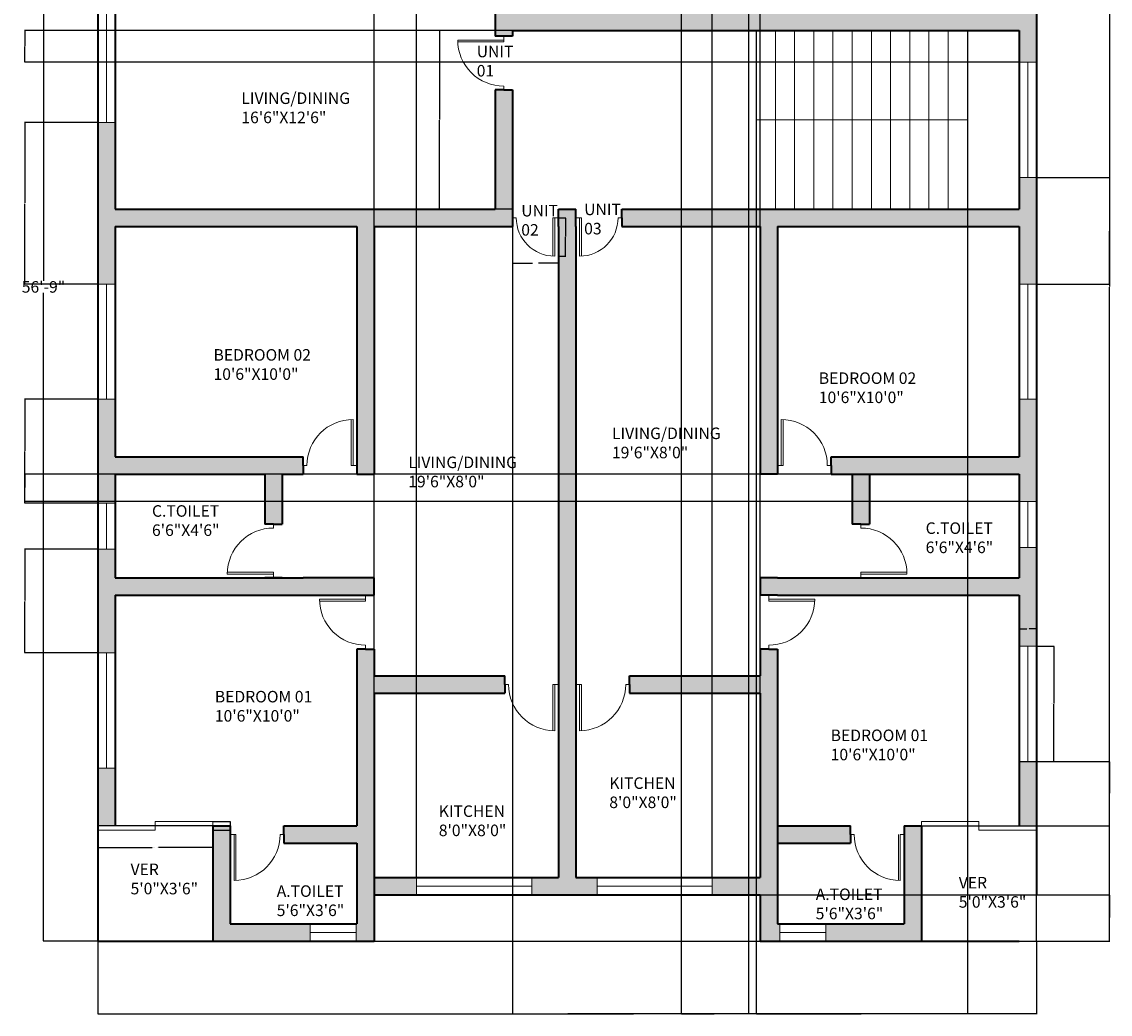
# Model space of a CAD drawing. Units: inches. Extents: x -17 to 550, y -704 to 87.
# Tile 1 of 2: x -17 to 550, y -704 to -187. Entities that reach past the tile are written whole.
import ezdxf

# ---------------------------------------------------------------- set-up
doc = ezdxf.new("R2010")
doc.units = ezdxf.units.IN
doc.header["$MEASUREMENT"] = 0
for name, color, linetype, lineweight in [('A-ANNO-DIMS', 2, 'Continuous', 18), ('A-AREA-IDEN', 7, 'Continuous', 18), ('A-DOOR', 3, 'Continuous', 18), ('A-FLOR-OTLN', 7, 'Continuous', 25), ('A-FLOR-STRS', 7, 'Continuous', 18), ('A-GLAZ', 4, 'Continuous', 18), ('A-WALL', 7, 'Continuous', 35), ('A-WALL-PATT', 252, 'Continuous', 13)]:
    doc.layers.add(name, color=color, linetype=linetype, lineweight=lineweight)
doc.styles.get("Standard").update_dxf_attribs({"font": 'arial.ttf'})
doc.dimstyles.get("Standard").update_dxf_attribs({"dimtxt": 0.18, "dimasz": 0.18, "dimexe": 0.18, "dimexo": 0.0625, "dimgap": 0.09, "dimtad": 0, "dimtih": 1, "dimtoh": 1, "dimdec": 0, "dimzin": 0, "dimdsep": 46, "dimlunit": 3, "dimtxsty": 'Standard', "dimcen": 0.09, "dimadec": 0, "dimazin": 0, "dimtfac": 1, "dimtdec": 0, "dimtofl": 0, "dimtmove": 0, "dimatfit": 3, "dimfxl": 1, "dimtolj": 1, "dimtzin": 0, "dimarcsym": 0})

# ---------------------------------------------------------------- blocks, each defined once
blk = doc.blocks.new('*D2')
at = {"layer": 'A-ANNO-DIMS', "color": 0, "lineweight": -2, "transparency": 16777216}
for p, q in [((22.68, 15.33), (-5.69, 15.33)), ((-5.51, 15.15), (-5.51, -322.02)), ((-5.51, -665.49), (-5.51, -328.33)), ((22.68, -665.67), (-5.69, -665.67))]:
    blk.add_line(p, q, dxfattribs=at)
at = {"layer": 'A-ANNO-DIMS', "color": 0, "transparency": 16777216}
for points in [[(-5.54, 15.15), (-5.48, 15.15), (-5.51, 15.33)], [(-5.54, -665.49), (-5.48, -665.49), (-5.51, -665.67)]]:
    blk.add_solid(points, dxfattribs=at)
at = {"layer": 'Defpoints', "color": 0, "transparency": 16777216}
for p in [(22.74, 15.33), (-5.51, -665.67), (22.74, -665.67)]:
    blk.add_point(p, dxfattribs=at)
at = {"layer": 'A-ANNO-DIMS', "color": 0, "transparency": 16777216, "insert": (-5.51, -325.17), "char_height": 6, "attachment_point": 5}
blk.add_mtext('\\A1;56\'-9"', dxfattribs=at)
blk = doc.blocks.new('WIN-60IN')
for p, q in [((0, 9), (60, 9)), ((0, 0), (0, 9)), ((60, 9), (60, 0)), ((0, 4.5), (60, 4.5)), ((60, 0), (0, 0))]:
    blk.add_line(p, q)
blk = doc.blocks.new('WIN-24IN')
for p, q in [((0, 24), (0, 0)), ((9, 24), (0, 24)), ((4.5, 24), (4.5, 0)), ((9, 0), (9, 24)), ((0, 0), (9, 0))]:
    blk.add_line(p, q)
blk = doc.blocks.new('DOOR-SWING-24IN')
for p, q in [((25, 0), (25, 24)), ((26, 0), (26, 24)), ((2, 0), (0, 0)), ((25, 0), (26, 0)), ((28, 0), (26, 0))]:
    blk.add_line(p, q)
blk.add_arc((26, 0), 24, 90, 180)
blk = doc.blocks.new('DOOR-SWING-20IN')
for p, q in [((0, 20), (2, 20)), ((21, 20), (21, 0)), ((21, 20), (22, 20)), ((22, 20), (22, 0)), ((24, 20), (22, 20))]:
    blk.add_line(p, q)
blk.add_arc((22, 20), 20, 180, 270)
blk = doc.blocks.new('DOOR-SLIDING-60IN')
for p, q in [((0, 0), (0, 2.25)), ((0, 2.25), (60, 2.25)), ((30, 4.5), (60, 4.5)), ((30, 2.25), (30, 4.5)), ((30, 2.25), (30, 0)), ((60, 4.5), (60, 2.25)), ((30, 0), (0, 0))]:
    blk.add_line(p, q)
blk = doc.blocks.new('*D10')
at = {"layer": 'A-ANNO-DIMS', "color": 0, "lineweight": -2, "transparency": 16777216}
for p, q in [((511.81, -512.17), (520.92, -512.17)), ((520.74, -512.35), (520.74, -541.99)), ((520.74, -571.99), (520.74, -542.36)), ((511.81, -572.17), (520.92, -572.17))]:
    blk.add_line(p, q, dxfattribs=at)
at = {"layer": 'A-ANNO-DIMS', "color": 0, "transparency": 16777216}
for points in [[(520.71, -512.35), (520.77, -512.35), (520.74, -512.17)], [(520.71, -571.99), (520.77, -571.99), (520.74, -572.17)]]:
    blk.add_solid(points, dxfattribs=at)
at = {"layer": 'Defpoints', "color": 0, "transparency": 16777216}
for p in [(511.74, -512.17), (520.74, -512.17), (511.74, -572.17)]:
    blk.add_point(p, dxfattribs=at)
at = {"layer": 'A-ANNO-DIMS', "color": 0, "transparency": 16777216, "insert": (520.74, -542.17), "char_height": 0.18, "attachment_point": 5}
blk.add_mtext('\\A1;WINDOW 5\'-0" TYP.', dxfattribs=at)
blk = doc.blocks.new('*D11')
at = {"layer": 'A-ANNO-DIMS', "color": 0, "lineweight": -2, "transparency": 16777216}
for p, q in [((502.74, -512.11), (502.74, -502.99)), ((502.92, -503.17), (506.6, -503.17)), ((511.56, -503.17), (507.88, -503.17)), ((511.74, -512.11), (511.74, -502.99))]:
    blk.add_line(p, q, dxfattribs=at)
at = {"layer": 'A-ANNO-DIMS', "color": 0, "transparency": 16777216}
for points in [[(502.92, -503.14), (502.92, -503.2), (502.74, -503.17)], [(511.56, -503.14), (511.56, -503.2), (511.74, -503.17)]]:
    blk.add_solid(points, dxfattribs=at)
at = {"layer": 'Defpoints', "color": 0, "transparency": 16777216}
for p in [(502.74, -503.17), (502.74, -512.17), (511.74, -512.17)]:
    blk.add_point(p, dxfattribs=at)
at = {"layer": 'A-ANNO-DIMS', "color": 0, "transparency": 16777216, "insert": (507.24, -503.17), "char_height": 0.18, "attachment_point": 5}
blk.add_mtext('\\A1;0\'-9" TYP.', dxfattribs=at)
blk = doc.blocks.new('*D14')
at = {"layer": 'A-ANNO-DIMS', "color": 0, "lineweight": -2, "transparency": 16777216}
for p, q in [((238.74, -309.24), (238.74, -312.95)), ((262.74, -309.24), (262.74, -312.95)), ((238.92, -312.77), (249.24, -312.77)), ((262.56, -312.77), (252.25, -312.77))]:
    blk.add_line(p, q, dxfattribs=at)
at = {"layer": 'A-ANNO-DIMS', "color": 0, "transparency": 16777216}
for points in [[(238.92, -312.74), (238.92, -312.8), (238.74, -312.77)], [(262.56, -312.74), (262.56, -312.8), (262.74, -312.77)]]:
    blk.add_solid(points, dxfattribs=at)
at = {"layer": 'Defpoints', "color": 0, "transparency": 16777216}
for p in [(238.74, -309.17), (262.74, -309.17), (262.74, -312.77)]:
    blk.add_point(p, dxfattribs=at)
at = {"layer": 'A-ANNO-DIMS', "color": 0, "transparency": 16777216, "insert": (250.74, -312.77), "char_height": 0.18, "attachment_point": 5}
blk.add_mtext('\\A1;ENTRY DOOR 2\'-0" TYP.', dxfattribs=at)
blk = doc.blocks.new('*D15')
at = {"layer": 'A-ANNO-DIMS', "color": 0, "lineweight": -2, "transparency": 16777216}
for p, q in [((262.81, -289.17), (266.52, -289.17)), ((266.34, -289.35), (266.34, -298.99)), ((266.34, -308.99), (266.34, -299.36)), ((262.81, -309.17), (266.52, -309.17))]:
    blk.add_line(p, q, dxfattribs=at)
at = {"layer": 'A-ANNO-DIMS', "color": 0, "transparency": 16777216}
for points in [[(266.31, -289.35), (266.37, -289.35), (266.34, -289.17)], [(266.31, -308.99), (266.37, -308.99), (266.34, -309.17)]]:
    blk.add_solid(points, dxfattribs=at)
at = {"layer": 'Defpoints', "color": 0, "transparency": 16777216}
for p in [(262.74, -289.17), (266.34, -289.17), (262.74, -309.17)]:
    blk.add_point(p, dxfattribs=at)
at = {"layer": 'A-ANNO-DIMS', "color": 0, "transparency": 16777216, "insert": (266.34, -299.17), "char_height": 0.18, "attachment_point": 5}
blk.add_mtext('\\A1;1\'-8" TYP.', dxfattribs=at)
blk = doc.blocks.new('*D16')
at = {"layer": 'A-ANNO-DIMS', "color": 0, "lineweight": -2, "transparency": 16777216}
for p, q in [((22.74, -607.99), (22.74, -617.1)), ((82.74, -607.99), (82.74, -617.1)), ((22.92, -616.92), (51.15, -616.92)), ((82.56, -616.92), (54.33, -616.92))]:
    blk.add_line(p, q, dxfattribs=at)
at = {"layer": 'A-ANNO-DIMS', "color": 0, "transparency": 16777216}
for points in [[(22.92, -616.89), (22.92, -616.95), (22.74, -616.92)], [(82.56, -616.89), (82.56, -616.95), (82.74, -616.92)]]:
    blk.add_solid(points, dxfattribs=at)
at = {"layer": 'Defpoints', "color": 0, "transparency": 16777216}
for p in [(22.74, -607.92), (82.74, -607.92), (82.74, -616.92)]:
    blk.add_point(p, dxfattribs=at)
at = {"layer": 'A-ANNO-DIMS', "color": 0, "transparency": 16777216, "insert": (52.74, -616.92), "char_height": 0.18, "attachment_point": 5}
blk.add_mtext('\\A1;SLIDING DOOR 5\'-0" TYP.', dxfattribs=at)
blk = doc.blocks.new('*D17')
at = {"layer": 'A-ANNO-DIMS', "color": 0, "lineweight": -2, "transparency": 16777216}
for p, q in [((82.81, -603.42), (91.92, -603.42)), ((91.74, -603.6), (91.74, -605.49)), ((91.74, -607.74), (91.74, -605.86)), ((82.81, -607.92), (91.92, -607.92))]:
    blk.add_line(p, q, dxfattribs=at)
at = {"layer": 'A-ANNO-DIMS', "color": 0, "transparency": 16777216}
for points in [[(91.71, -603.6), (91.77, -603.6), (91.74, -603.42)], [(91.71, -607.74), (91.77, -607.74), (91.74, -607.92)]]:
    blk.add_solid(points, dxfattribs=at)
at = {"layer": 'Defpoints', "color": 0, "transparency": 16777216}
for p in [(82.74, -603.42), (91.74, -603.42), (82.74, -607.92)]:
    blk.add_point(p, dxfattribs=at)
at = {"layer": 'A-ANNO-DIMS', "color": 0, "transparency": 16777216, "insert": (91.74, -605.67), "char_height": 0.18, "attachment_point": 5}
blk.add_mtext('\\A1;0\'-4 1/2" TYP.', dxfattribs=at)
blk = doc.blocks.new('*D18')
at = {"layer": 'A-ANNO-DIMS', "color": 0, "lineweight": -2, "transparency": 16777216}
for p, q in [((22.74, -665.74), (22.74, -703.75)), ((511.74, -665.74), (511.74, -703.75)), ((22.92, -703.57), (266.84, -703.57)), ((511.56, -703.57), (267.65, -703.57))]:
    blk.add_line(p, q, dxfattribs=at)
at = {"layer": 'A-ANNO-DIMS', "color": 0, "transparency": 16777216}
for points in [[(22.92, -703.54), (22.92, -703.6), (22.74, -703.57)], [(511.56, -703.54), (511.56, -703.6), (511.74, -703.57)]]:
    blk.add_solid(points, dxfattribs=at)
at = {"layer": 'Defpoints', "color": 0, "transparency": 16777216}
for p in [(22.74, -665.67), (511.74, -665.67), (511.74, -703.57)]:
    blk.add_point(p, dxfattribs=at)
at = {"layer": 'A-ANNO-DIMS', "color": 0, "transparency": 16777216, "insert": (267.24, -703.57), "char_height": 0.18, "attachment_point": 5}
blk.add_mtext('\\A1;40\'-9"', dxfattribs=at)
blk = doc.blocks.new('*D19')
at = {"layer": 'A-ANNO-DIMS', "color": 0, "lineweight": -2, "transparency": 16777216}
for p, q in [((238.68, -191.67), (200.66, -191.67)), ((200.84, -191.85), (200.84, -237.99)), ((200.84, -284.49), (200.84, -238.36)), ((238.68, -284.67), (200.66, -284.67))]:
    blk.add_line(p, q, dxfattribs=at)
at = {"layer": 'A-ANNO-DIMS', "color": 0, "transparency": 16777216}
for points in [[(200.81, -191.85), (200.87, -191.85), (200.84, -191.67)], [(200.81, -284.49), (200.87, -284.49), (200.84, -284.67)]]:
    blk.add_solid(points, dxfattribs=at)
at = {"layer": 'Defpoints', "color": 0, "transparency": 16777216}
for p in [(200.84, -191.67), (238.74, -191.67), (238.74, -284.67)]:
    blk.add_point(p, dxfattribs=at)
at = {"layer": 'A-ANNO-DIMS', "color": 0, "transparency": 16777216, "insert": (200.84, -238.17), "char_height": 0.18, "attachment_point": 5}
blk.add_mtext('\\A1;7\'-9"', dxfattribs=at)
blk = doc.blocks.new('*D20')
at = {"layer": 'A-ANNO-DIMS', "color": 0, "lineweight": -2, "transparency": 16777216}
for p, q in [((365.68, -191.74), (365.68, -703.75)), ((475.68, -191.74), (475.68, -703.75)), ((365.86, -703.57), (420.35, -703.57)), ((475.5, -703.57), (421.01, -703.57))]:
    blk.add_line(p, q, dxfattribs=at)
at = {"layer": 'A-ANNO-DIMS', "color": 0, "transparency": 16777216}
for points in [[(365.86, -703.54), (365.86, -703.6), (365.68, -703.57)], [(475.5, -703.54), (475.5, -703.6), (475.68, -703.57)]]:
    blk.add_solid(points, dxfattribs=at)
at = {"layer": 'Defpoints', "color": 0, "transparency": 16777216}
for p in [(365.68, -191.67), (475.68, -191.67), (475.68, -703.57)]:
    blk.add_point(p, dxfattribs=at)
at = {"layer": 'A-ANNO-DIMS', "color": 0, "transparency": 16777216, "insert": (420.68, -703.57), "char_height": 0.18, "attachment_point": 5}
blk.add_mtext('\\A1;9\'-2"', dxfattribs=at)
blk = doc.blocks.new('*D21')
at = {"layer": 'A-ANNO-DIMS', "color": 0, "lineweight": -2, "transparency": 16777216}
for p, q in [((238.74, -222.74), (238.74, -703.75)), ((365.68, -238.24), (365.68, -703.75)), ((238.92, -703.57), (301.82, -703.57)), ((365.5, -703.57), (302.6, -703.57))]:
    blk.add_line(p, q, dxfattribs=at)
at = {"layer": 'A-ANNO-DIMS', "color": 0, "transparency": 16777216}
for points in [[(238.92, -703.54), (238.92, -703.6), (238.74, -703.57)], [(365.5, -703.54), (365.5, -703.6), (365.68, -703.57)]]:
    blk.add_solid(points, dxfattribs=at)
at = {"layer": 'Defpoints', "color": 0, "transparency": 16777216}
for p in [(238.74, -222.67), (365.68, -238.17), (365.68, -703.57)]:
    blk.add_point(p, dxfattribs=at)
at = {"layer": 'A-ANNO-DIMS', "color": 0, "transparency": 16777216, "insert": (302.21, -703.57), "char_height": 0.18, "attachment_point": 5}
blk.add_mtext('\\A1;10\'-7"', dxfattribs=at)
blk = doc.blocks.new('*D22')
at = {"layer": 'A-ANNO-DIMS', "color": 0, "lineweight": -2, "transparency": 16777216}
for p, q in [((166.81, -641.67), (549.82, -641.67)), ((549.64, -641.85), (549.64, -653.49)), ((549.64, -665.49), (549.64, -653.86)), ((166.81, -665.67), (549.82, -665.67))]:
    blk.add_line(p, q, dxfattribs=at)
at = {"layer": 'A-ANNO-DIMS', "color": 0, "transparency": 16777216}
for points in [[(549.61, -641.85), (549.67, -641.85), (549.64, -641.67)], [(549.61, -665.49), (549.67, -665.49), (549.64, -665.67)]]:
    blk.add_solid(points, dxfattribs=at)
at = {"layer": 'Defpoints', "color": 0, "transparency": 16777216}
for p in [(166.74, -641.67), (549.64, -641.67), (166.74, -665.67)]:
    blk.add_point(p, dxfattribs=at)
at = {"layer": 'A-ANNO-DIMS', "color": 0, "transparency": 16777216, "insert": (549.64, -653.67), "char_height": 0.18, "attachment_point": 5}
blk.add_mtext('\\A1;2\'-0"', dxfattribs=at)
blk = doc.blocks.new('*D29')
at = {"layer": 'A-ANNO-DIMS', "color": 0, "lineweight": -2, "transparency": 16777216}
for p, q in [((22.68, -239.67), (-15.34, -239.67)), ((-15.16, -239.85), (-15.16, -281.49)), ((-15.16, -323.49), (-15.16, -281.86)), ((22.68, -323.67), (-15.34, -323.67))]:
    blk.add_line(p, q, dxfattribs=at)
at = {"layer": 'A-ANNO-DIMS', "color": 0, "transparency": 16777216}
for points in [[(-15.19, -239.85), (-15.13, -239.85), (-15.16, -239.67)], [(-15.19, -323.49), (-15.13, -323.49), (-15.16, -323.67)]]:
    blk.add_solid(points, dxfattribs=at)
at = {"layer": 'Defpoints', "color": 0, "transparency": 16777216}
for p in [(-15.16, -239.67), (22.74, -239.67), (22.74, -323.67)]:
    blk.add_point(p, dxfattribs=at)
at = {"layer": 'A-ANNO-DIMS', "color": 0, "transparency": 16777216, "insert": (-15.16, -281.67), "char_height": 0.18, "attachment_point": 5}
blk.add_mtext('\\A1;7\'-0"', dxfattribs=at)
blk = doc.blocks.new('*D30')
at = {"layer": 'A-ANNO-DIMS', "color": 0, "lineweight": -2, "transparency": 16777216}
for p, q in [((22.68, -383.67), (-15.34, -383.67)), ((-15.16, -383.85), (-15.16, -410.49)), ((-15.16, -437.49), (-15.16, -410.86)), ((22.68, -437.67), (-15.34, -437.67))]:
    blk.add_line(p, q, dxfattribs=at)
at = {"layer": 'A-ANNO-DIMS', "color": 0, "transparency": 16777216}
for points in [[(-15.19, -383.85), (-15.13, -383.85), (-15.16, -383.67)], [(-15.19, -437.49), (-15.13, -437.49), (-15.16, -437.67)]]:
    blk.add_solid(points, dxfattribs=at)
at = {"layer": 'Defpoints', "color": 0, "transparency": 16777216}
for p in [(-15.16, -383.67), (22.74, -383.67), (22.74, -437.67)]:
    blk.add_point(p, dxfattribs=at)
at = {"layer": 'A-ANNO-DIMS', "color": 0, "transparency": 16777216, "insert": (-15.16, -410.67), "char_height": 0.18, "attachment_point": 5}
blk.add_mtext('\\A1;4\'-6"', dxfattribs=at)
blk = doc.blocks.new('*D31')
at = {"layer": 'A-ANNO-DIMS', "color": 0, "lineweight": -2, "transparency": 16777216}
for p, q in [((22.68, -461.67), (-15.34, -461.67)), ((-15.16, -461.85), (-15.16, -488.49)), ((-15.16, -515.49), (-15.16, -488.86)), ((22.68, -515.67), (-15.34, -515.67))]:
    blk.add_line(p, q, dxfattribs=at)
at = {"layer": 'A-ANNO-DIMS', "color": 0, "transparency": 16777216}
for points in [[(-15.19, -461.85), (-15.13, -461.85), (-15.16, -461.67)], [(-15.19, -515.49), (-15.13, -515.49), (-15.16, -515.67)]]:
    blk.add_solid(points, dxfattribs=at)
at = {"layer": 'Defpoints', "color": 0, "transparency": 16777216}
for p in [(-15.16, -461.67), (22.74, -461.67), (22.74, -515.67)]:
    blk.add_point(p, dxfattribs=at)
at = {"layer": 'A-ANNO-DIMS', "color": 0, "transparency": 16777216, "insert": (-15.16, -488.67), "char_height": 0.18, "attachment_point": 5}
blk.add_mtext('\\A1;4\'-6"', dxfattribs=at)
blk = doc.blocks.new('*D32')
at = {"layer": 'A-ANNO-DIMS', "color": 0, "lineweight": -2, "transparency": 16777216}
for p, q in [((326.67, -134.74), (326.67, -703.75)), ((361.74, -134.74), (361.74, -703.75)), ((326.85, -703.57), (343.81, -703.57)), ((361.56, -703.57), (344.61, -703.57))]:
    blk.add_line(p, q, dxfattribs=at)
at = {"layer": 'A-ANNO-DIMS', "color": 0, "transparency": 16777216}
for points in [[(326.85, -703.54), (326.85, -703.6), (326.67, -703.57)], [(361.56, -703.54), (361.56, -703.6), (361.74, -703.57)]]:
    blk.add_solid(points, dxfattribs=at)
at = {"layer": 'Defpoints', "color": 0, "transparency": 16777216}
for p in [(326.67, -134.67), (361.74, -134.67), (361.74, -703.57)]:
    blk.add_point(p, dxfattribs=at)
at = {"layer": 'A-ANNO-DIMS', "color": 0, "transparency": 16777216, "insert": (344.21, -703.57), "char_height": 0.18, "attachment_point": 5}
blk.add_mtext('\\A1;2\'-11"', dxfattribs=at)
blk = doc.blocks.new('*D33')
at = {"layer": 'A-ANNO-DIMS', "color": 0, "lineweight": -2, "transparency": 16777216}
for p, q in [((166.74, -632.61), (166.74, 53.41)), ((166.92, 53.23), (177.41, 53.23)), ((188.68, 53.23), (178.19, 53.23)), ((188.86, -632.61), (188.86, 53.41))]:
    blk.add_line(p, q, dxfattribs=at)
at = {"layer": 'A-ANNO-DIMS', "color": 0, "transparency": 16777216}
for points in [[(166.92, 53.26), (166.92, 53.2), (166.74, 53.23)], [(188.68, 53.26), (188.68, 53.2), (188.86, 53.23)]]:
    blk.add_solid(points, dxfattribs=at)
at = {"layer": 'Defpoints', "color": 0, "transparency": 16777216}
for p in [(188.86, 53.23), (166.74, -632.67), (188.86, -632.67)]:
    blk.add_point(p, dxfattribs=at)
at = {"layer": 'A-ANNO-DIMS', "color": 0, "transparency": 16777216, "insert": (177.8, 53.23), "char_height": 0.18, "attachment_point": 5}
blk.add_mtext('\\A1;1\'-10"', dxfattribs=at)
blk = doc.blocks.new('*D34')
at = {"layer": 'A-ANNO-DIMS', "color": 0, "lineweight": -2, "transparency": 16777216}
for p, q in [((342.82, -632.61), (342.82, 53.41)), ((343, 53.23), (354.95, 53.23)), ((367.56, 53.23), (355.61, 53.23)), ((367.74, -632.61), (367.74, 53.41))]:
    blk.add_line(p, q, dxfattribs=at)
at = {"layer": 'A-ANNO-DIMS', "color": 0, "transparency": 16777216}
for points in [[(343, 53.26), (343, 53.2), (342.82, 53.23)], [(367.56, 53.26), (367.56, 53.2), (367.74, 53.23)]]:
    blk.add_solid(points, dxfattribs=at)
at = {"layer": 'Defpoints', "color": 0, "transparency": 16777216}
for p in [(367.74, 53.23), (342.82, -632.67), (367.74, -632.67)]:
    blk.add_point(p, dxfattribs=at)
at = {"layer": 'A-ANNO-DIMS', "color": 0, "transparency": 16777216, "insert": (355.28, 53.23), "char_height": 0.18, "attachment_point": 5}
blk.add_mtext('\\A1;2\'-1"', dxfattribs=at)
blk = doc.blocks.new('*D35')
at = {"layer": 'A-ANNO-DIMS', "color": 0, "lineweight": -2, "transparency": 16777216}
for p, q in [((502.68, -191.67), (-15.34, -191.67)), ((-15.16, -191.85), (-15.16, -199.74)), ((-15.16, -207.99), (-15.16, -200.11)), ((502.68, -208.17), (-15.34, -208.17))]:
    blk.add_line(p, q, dxfattribs=at)
at = {"layer": 'A-ANNO-DIMS', "color": 0, "transparency": 16777216}
for points in [[(-15.19, -191.85), (-15.13, -191.85), (-15.16, -191.67)], [(-15.19, -207.99), (-15.13, -207.99), (-15.16, -208.17)]]:
    blk.add_solid(points, dxfattribs=at)
at = {"layer": 'Defpoints', "color": 0, "transparency": 16777216}
for p in [(502.74, -191.67), (-15.16, -208.17), (502.74, -208.17)]:
    blk.add_point(p, dxfattribs=at)
at = {"layer": 'A-ANNO-DIMS', "color": 0, "transparency": 16777216, "insert": (-15.16, -199.92), "char_height": 0.18, "attachment_point": 5}
blk.add_mtext('\\A1;1\'-4 1/2"', dxfattribs=at)
blk = doc.blocks.new('*D36')
at = {"layer": 'A-ANNO-DIMS', "color": 0, "lineweight": -2, "transparency": 16777216}
for p, q in [((511.81, -268.17), (549.82, -268.17)), ((549.64, -268.35), (549.64, -295.74)), ((549.64, -323.49), (549.64, -296.11)), ((511.81, -323.67), (549.82, -323.67))]:
    blk.add_line(p, q, dxfattribs=at)
at = {"layer": 'A-ANNO-DIMS', "color": 0, "transparency": 16777216}
for points in [[(549.61, -268.35), (549.67, -268.35), (549.64, -268.17)], [(549.61, -323.49), (549.67, -323.49), (549.64, -323.67)]]:
    blk.add_solid(points, dxfattribs=at)
at = {"layer": 'Defpoints', "color": 0, "transparency": 16777216}
for p in [(511.74, -268.17), (511.74, -323.67), (549.64, -323.67)]:
    blk.add_point(p, dxfattribs=at)
at = {"layer": 'A-ANNO-DIMS', "color": 0, "transparency": 16777216, "insert": (549.64, -295.92), "char_height": 0.18, "attachment_point": 5}
blk.add_mtext('\\A1;4\'-7 1/2"', dxfattribs=at)
blk = doc.blocks.new('*D37')
at = {"layer": 'A-ANNO-DIMS', "color": 0, "lineweight": -2, "transparency": 16777216}
for p, q in [((502.68, -422.67), (-15.34, -422.67)), ((-15.16, -422.85), (-15.16, -429.57)), ((-15.16, -436.64), (-15.16, -429.93)), ((502.68, -436.82), (-15.34, -436.82))]:
    blk.add_line(p, q, dxfattribs=at)
at = {"layer": 'A-ANNO-DIMS', "color": 0, "transparency": 16777216}
for points in [[(-15.19, -422.85), (-15.13, -422.85), (-15.16, -422.67)], [(-15.19, -436.64), (-15.13, -436.64), (-15.16, -436.82)]]:
    blk.add_solid(points, dxfattribs=at)
at = {"layer": 'Defpoints', "color": 0, "transparency": 16777216}
for p in [(502.74, -422.67), (-15.16, -436.82), (502.74, -436.82)]:
    blk.add_point(p, dxfattribs=at)
at = {"layer": 'A-ANNO-DIMS', "color": 0, "transparency": 16777216, "insert": (-15.16, -429.75), "char_height": 0.18, "attachment_point": 5}
blk.add_mtext('\\A1;1\'-2"', dxfattribs=at)
blk = doc.blocks.new('*D38')
at = {"layer": 'A-ANNO-DIMS', "color": 0, "lineweight": -2, "transparency": 16777216}
for p, q in [((502.81, -572.17), (549.82, -572.17)), ((549.64, -572.35), (549.64, -588.74)), ((549.64, -605.49), (549.64, -589.11)), ((502.81, -605.67), (549.82, -605.67))]:
    blk.add_line(p, q, dxfattribs=at)
at = {"layer": 'A-ANNO-DIMS', "color": 0, "transparency": 16777216}
for points in [[(549.61, -572.35), (549.67, -572.35), (549.64, -572.17)], [(549.61, -605.49), (549.67, -605.49), (549.64, -605.67)]]:
    blk.add_solid(points, dxfattribs=at)
at = {"layer": 'Defpoints', "color": 0, "transparency": 16777216}
for p in [(502.74, -572.17), (502.74, -605.67), (549.64, -605.67)]:
    blk.add_point(p, dxfattribs=at)
at = {"layer": 'A-ANNO-DIMS', "color": 0, "transparency": 16777216, "insert": (549.64, -588.92), "char_height": 0.18, "attachment_point": 5}
blk.add_mtext('\\A1;2\'-9 1/2"', dxfattribs=at)
blk = doc.blocks.new('*D41')
at = {"layer": 'A-ANNO-DIMS', "color": 0, "lineweight": -2, "transparency": 16777216}
for p, q in [((475.81, 15.33), (549.82, 15.33)), ((549.64, 15.15), (549.64, -324.99)), ((549.64, -665.49), (549.64, -325.36)), ((511.81, -665.67), (549.82, -665.67))]:
    blk.add_line(p, q, dxfattribs=at)
at = {"layer": 'A-ANNO-DIMS', "color": 0, "transparency": 16777216}
for points in [[(549.61, 15.15), (549.67, 15.15), (549.64, 15.33)], [(549.61, -665.49), (549.67, -665.49), (549.64, -665.67)]]:
    blk.add_solid(points, dxfattribs=at)
at = {"layer": 'Defpoints', "color": 0, "transparency": 16777216}
for p in [(475.74, 15.33), (549.64, 15.33), (511.74, -665.67)]:
    blk.add_point(p, dxfattribs=at)
at = {"layer": 'A-ANNO-DIMS', "color": 0, "transparency": 16777216, "insert": (549.64, -325.17), "char_height": 0.18, "attachment_point": 5}
blk.add_mtext('\\A1;56\'-9"', dxfattribs=at)

msp = doc.modelspace()

# ---------------------------------------------------------------- hatches: boundary and pattern name
at = {"layer": 'A-WALL-PATT'}
h = msp.add_hatch(color=256, dxfattribs=at)
h.dxf.hatch_style = 1
h.paths.add_polyline_path([(322.74, 6.33), (364.74, 6.33), (364.74, 15.33), (307.74, 15.33), (307.74, 6.33), (313.74, 6.33), (313.74, -77.67), (269.74, -77.67), (269.74, -82.17), (269.74, -86.67), (322.74, -86.67)])
h.paths.add_polyline_path([(475.74, 15.33), (424.74, 15.33), (424.74, 6.33), (466.74, 6.33), (466.74, -29.67), (475.74, -29.67)])
h.paths.add_polyline_path([(475.74, -89.67), (466.74, -89.67), (466.74, -125.67), (398.74, -125.67), (398.74, -130.17), (398.74, -134.67), (466.74, -134.67), (466.74, -146.67), (475.74, -146.67)])
h.paths.add_polyline_path([(511.74, -182.67), (475.74, -182.67), (475.74, -170.67), (466.74, -170.67), (466.74, -182.67), (370.74, -182.67), (370.74, -134.67), (370.74, -125.67), (313.74, -125.67), (313.74, -134.67), (361.74, -134.67), (361.74, -182.67), (229.74, -182.67), (229.74, -194.67), (238.74, -194.67), (238.74, -191.67), (502.74, -191.67), (502.74, -208.17), (511.74, -208.17)])
h.paths.add_polyline_path([(184.74, -86.67), (204.74, -86.67), (204.74, -82.17), (204.74, -77.67), (184.74, -77.67), (184.74, 6.33), (208.53, 6.33), (208.53, 15.33), (133.74, 15.33), (133.74, 6.33), (175.74, 6.33), (175.74, -134.67), (184.74, -134.67)])
h.paths.add_polyline_path([(241.74, 6.33), (247.74, 6.33), (247.74, 15.33), (232.53, 15.33), (232.53, 6.33), (232.74, 6.33), (232.74, -86.67), (241.74, -86.67)])
h.paths.add_polyline_path([(147.74, -125.67), (31.74, -125.67), (31.74, -89.67), (22.74, -89.67), (22.74, -179.67), (31.74, -179.67), (31.74, -134.67), (147.74, -134.67), (147.74, -130.17)])
h.paths.add_polyline_path([(31.74, 6.33), (73.74, 6.33), (73.74, 15.33), (22.74, 15.33), (22.74, -29.67), (31.74, -29.67)])
h.paths.add_polyline_path([(238.74, -284.67), (238.74, -222.67), (234.24, -222.67), (229.74, -222.67), (229.74, -284.67), (31.74, -284.67), (31.74, -239.67), (22.74, -239.67), (22.74, -323.67), (31.74, -323.67), (31.74, -293.67), (157.74, -293.67), (157.74, -422.67), (166.74, -422.67), (166.74, -293.67), (238.74, -293.67)])
h.paths.add_polyline_path([(511.74, -268.17), (502.74, -268.17), (502.74, -284.67), (370.74, -284.67), (361.74, -284.67), (295.74, -284.67), (295.74, -289.17), (295.74, -293.67), (367.74, -293.67), (367.74, -422.67), (376.74, -422.67), (376.74, -413.67), (376.74, -293.67), (502.74, -293.67), (502.74, -323.67), (511.74, -323.67)])
h.paths.add_polyline_path([(511.74, -383.67), (502.74, -383.67), (502.74, -413.67), (404.74, -413.67), (404.74, -418.17), (404.74, -422.67), (502.74, -422.67), (502.74, -436.82), (511.74, -436.82)])
h.paths.add_polyline_path([(424.74, -422.67), (415.74, -422.67), (415.74, -448.67), (420.24, -448.67), (424.74, -448.67)])
h.paths.add_polyline_path([(511.74, -460.82), (502.74, -460.82), (502.74, -476.67), (376.74, -476.67), (367.74, -476.67), (367.74, -485.67), (376.74, -485.67), (502.74, -485.67), (502.74, -512.17), (511.74, -512.17)])
h.paths.add_polyline_path([(376.74, -513.67), (372.24, -513.67), (367.74, -513.67), (367.74, -527.67), (299.74, -527.67), (299.74, -532.17), (299.74, -536.67), (367.74, -536.67), (367.74, -632.67), (342.82, -632.67), (342.82, -641.67), (367.74, -641.67), (367.74, -665.67), (376.74, -665.67), (378.02, -665.67), (378.02, -656.67), (376.74, -656.67), (376.74, -614.67)])
h.paths.add_polyline_path([(511.74, -572.17), (502.74, -572.17), (502.74, -605.67), (511.74, -605.67)])
h.paths.add_polyline_path([(451.74, -605.67), (442.74, -605.67), (442.74, -656.67), (402.02, -656.67), (402.02, -665.67), (451.74, -665.67)])
h.paths.add_polyline_path([(414.74, -605.67), (376.74, -605.67), (376.74, -614.67), (414.74, -614.67), (414.74, -610.17)])
h.paths.add_polyline_path([(282.82, -632.67), (271.74, -632.67), (271.74, -293.67), (271.74, -284.67), (262.74, -284.67), (262.74, -293.67), (262.74, -632.67), (248.86, -632.67), (248.86, -641.67), (282.82, -641.67)])
h.paths.add_polyline_path([(166.74, -536.67), (234.74, -536.67), (234.74, -532.17), (234.74, -527.67), (166.74, -527.67), (166.74, -513.67), (162.24, -513.67), (157.74, -513.67), (157.74, -605.67), (119.74, -605.67), (119.74, -610.17), (119.74, -614.67), (157.74, -614.67), (157.74, -656.67), (157.43, -665.67), (166.74, -665.67)])
h.paths.add_polyline_path([(188.86, -632.67), (166.74, -632.67), (166.74, -641.67), (188.86, -641.67)], flags=17)
h.paths.add_polyline_path([(133.43, -656.67), (91.74, -656.67), (91.74, -605.67), (82.74, -605.67), (82.74, -665.67), (133.43, -665.67)])
h.paths.add_polyline_path([(31.74, -575.67), (22.74, -575.67), (22.74, -605.67), (31.74, -605.67)])
h.paths.add_polyline_path([(166.74, -476.67), (129.74, -476.67), (31.74, -476.67), (31.74, -461.67), (22.74, -461.67), (22.74, -515.67), (31.74, -515.67), (31.74, -485.67), (157.74, -485.67), (166.74, -485.67)])
h.paths.add_polyline_path([(129.74, -413.67), (31.74, -413.67), (31.74, -383.67), (22.74, -383.67), (22.74, -437.67), (31.74, -437.67), (31.74, -422.67), (109.74, -422.67), (109.74, -448.67), (114.24, -448.67), (118.74, -448.67), (118.74, -422.67), (129.74, -422.67), (129.74, -418.17)])

# ---------------------------------------------------------------- linework, layer by layer
at = {"layer": 'A-DOOR'}
for p, q in [((416.74, -610.17), (414.74, -610.17)), ((439.74, -610.17), (439.74, -634.17)), ((442.74, -610.17), (440.74, -610.17)), ((440.74, -610.17), (440.74, -634.17))]:
    msp.add_line(p, q, dxfattribs=at)
msp.add_arc((440.74, -610.17), 24, 180, 270, dxfattribs=at)
at = {"layer": 'A-FLOR-OTLN'}
for p, q in [((82.74, -605.67), (22.74, -605.67)), ((451.74, -605.67), (511.74, -605.67)), ((511.74, -665.67), (511.74, -641.67)), ((502.74, -665.67), (511.74, -665.67))]:
    msp.add_line(p, q, dxfattribs=at)
at = {"layer": 'A-FLOR-STRS'}
for p, q in [((365.68, -191.67), (365.68, -284.67)), ((375.68, -191.67), (375.68, -284.67)), ((385.68, -191.67), (385.68, -284.67)), ((395.68, -191.67), (395.68, -284.67)), ((405.68, -191.67), (405.68, -284.67)), ((415.68, -191.67), (415.68, -284.67)), ((425.68, -191.67), (425.68, -284.67)), ((435.68, -191.67), (435.68, -284.67)), ((445.68, -191.67), (445.68, -284.67)), ((455.68, -191.67), (455.68, -284.67)), ((465.68, -191.67), (465.68, -284.67)), ((475.68, -191.67), (475.68, -284.67)), ((365.68, -238.17), (475.68, -238.17))]:
    msp.add_line(p, q, dxfattribs=at)
at = {"layer": 'A-WALL'}
for p, q in [((22.74, 15.33), (22.74, -665.67)), ((31.74, -134.67), (31.74, -284.67)), ((229.74, -182.67), (229.74, -194.67)), ((511.74, -182.67), (511.74, -641.67)), ((238.74, -191.67), (466.74, -191.67)), ((238.74, -191.67), (238.74, -194.67)), ((238.74, -191.67), (502.74, -191.67)), ((502.74, -191.67), (502.74, -284.67)), ((238.74, -194.67), (229.74, -194.67)), ((234.24, -222.67), (229.74, -222.67)), ((229.74, -222.67), (229.74, -284.67)), ((234.24, -222.67), (238.74, -222.67)), ((238.74, -222.67), (238.74, -284.67)), ((31.74, -284.67), (229.74, -284.67)), ((238.74, -284.67), (238.74, -293.67)), ((262.74, -284.67), (271.74, -284.67)), ((262.74, -293.67), (262.74, -284.67)), ((271.74, -293.67), (271.74, -284.67)), ((295.74, -289.17), (295.74, -284.67)), ((295.74, -284.67), (361.74, -284.67)), ((361.74, -284.67), (370.74, -284.67)), ((370.74, -284.67), (502.74, -284.67)), ((31.74, -293.67), (157.74, -293.67)), ((31.74, -293.67), (31.74, -413.67)), ((157.74, -293.67), (157.74, -422.67)), ((166.74, -293.67), (166.74, -422.67)), ((166.74, -293.67), (238.74, -293.67)), ((262.74, -293.67), (262.74, -632.67)), ((271.74, -293.67), (271.74, -632.67)), ((295.74, -289.17), (295.74, -293.67)), ((295.74, -293.67), (367.74, -293.67)), ((367.74, -293.67), (367.74, -422.67)), ((376.74, -293.67), (376.74, -413.67)), ((376.74, -293.67), (502.74, -293.67)), ((502.74, -293.67), (502.74, -413.67)), ((31.74, -413.67), (129.74, -413.67)), ((129.74, -418.17), (129.74, -413.67)), ((376.74, -413.67), (376.74, -422.67)), ((404.74, -418.17), (404.74, -413.67)), ((404.74, -413.67), (502.74, -413.67)), ((129.74, -418.17), (129.74, -422.67)), ((404.74, -418.17), (404.74, -422.67)), ((31.74, -422.67), (109.74, -422.67)), ((31.74, -422.67), (31.74, -476.67)), ((109.74, -422.67), (109.74, -448.67)), ((118.74, -422.67), (118.74, -448.67)), ((118.74, -422.67), (129.74, -422.67)), ((157.74, -422.67), (166.74, -422.67)), ((376.74, -422.67), (367.74, -422.67)), ((404.74, -422.67), (502.74, -422.67)), ((415.74, -422.67), (415.74, -448.67)), ((424.74, -422.67), (424.74, -448.67)), ((502.74, -422.67), (502.74, -476.67)), ((114.24, -448.67), (109.74, -448.67)), ((114.24, -448.67), (118.74, -448.67)), ((420.24, -448.67), (415.74, -448.67)), ((420.24, -448.67), (424.74, -448.67)), ((31.74, -476.67), (129.74, -476.67)), ((118.74, -476.67), (109.74, -476.67)), ((166.74, -476.67), (129.74, -476.67)), ((166.74, -485.67), (166.74, -476.67)), ((376.74, -476.67), (367.74, -476.67)), ((367.74, -476.67), (367.74, -485.67)), ((376.74, -476.67), (502.74, -476.67)), ((31.74, -485.67), (157.74, -485.67)), ((31.74, -485.67), (31.74, -605.67)), ((157.74, -485.67), (166.74, -485.67)), ((376.74, -485.67), (367.74, -485.67)), ((376.74, -485.67), (502.74, -485.67)), ((502.74, -485.67), (502.74, -605.67)), ((162.24, -513.67), (157.74, -513.67)), ((157.74, -513.67), (157.74, -605.67)), ((162.24, -513.67), (166.74, -513.67)), ((166.74, -513.67), (166.74, -527.67)), ((372.24, -513.67), (367.74, -513.67)), ((367.74, -513.67), (367.74, -527.67)), ((372.24, -513.67), (376.74, -513.67)), ((376.74, -513.67), (376.74, -614.67)), ((166.74, -527.67), (234.74, -527.67)), ((234.74, -532.17), (234.74, -527.67)), ((234.74, -532.17), (234.74, -536.67)), ((299.74, -527.67), (367.74, -527.67)), ((299.74, -532.17), (299.74, -527.67)), ((299.74, -532.17), (299.74, -536.67)), ((166.74, -536.67), (234.74, -536.67)), ((166.74, -536.67), (166.74, -665.67)), ((299.74, -536.67), (367.74, -536.67)), ((367.74, -536.67), (367.74, -632.67)), ((82.74, -605.67), (91.74, -605.67)), ((82.74, -605.67), (82.74, -665.67)), ((91.74, -605.67), (91.74, -656.67)), ((119.74, -610.17), (119.74, -605.67)), ((119.74, -605.67), (157.74, -605.67)), ((376.74, -605.67), (414.74, -605.67)), ((414.74, -610.17), (414.74, -605.67)), ((442.74, -605.67), (442.74, -656.67)), ((442.74, -605.67), (451.74, -605.67)), ((451.74, -605.67), (451.74, -665.67)), ((119.74, -610.17), (119.74, -614.67)), ((414.74, -610.17), (414.74, -614.67)), ((119.74, -614.67), (157.74, -614.67)), ((157.74, -614.67), (157.74, -656.67)), ((376.74, -614.67), (414.74, -614.67)), ((376.74, -614.67), (376.74, -656.67)), ((166.74, -632.67), (262.74, -632.67)), ((271.74, -632.67), (367.74, -632.67)), ((166.74, -641.67), (367.74, -641.67)), ((367.74, -641.67), (367.74, -665.67)), ((91.74, -656.67), (157.74, -656.67)), ((376.74, -656.67), (442.74, -656.67)), ((22.74, -665.67), (166.74, -665.67)), ((367.74, -665.67), (376.74, -665.67)), ((376.74, -665.67), (502.74, -665.67))]:
    msp.add_line(p, q, dxfattribs=at)

# ---------------------------------------------------------------- block references
at = {"layer": 'A-DOOR'}
for p, rotation in [((234.24, -222.67), 90.00000000000018), ((420.24, -448.67), 269.9999999999996), ((162.24, -513.67), 90.00000000000018), ((299.74, -532.17), 180), ((119.74, -610.17), 180)]:
    msp.add_blockref('DOOR-SWING-24IN', p, dxfattribs=dict(at, rotation=rotation))
for name, p in [('DOOR-SWING-20IN', (238.74, -309.17)), ('DOOR-SWING-24IN', (129.74, -418.17)), ('DOOR-SLIDING-60IN', (22.74, -607.92))]:
    msp.add_blockref(name, p, dxfattribs=at)
at = {"layer": 'A-DOOR', "extrusion": (0, 0, -1), "zscale": -1}
for name, p in [('DOOR-SWING-20IN', (-295.74, -309.17)), ('DOOR-SWING-24IN', (-404.74, -418.17)), ('DOOR-SLIDING-60IN', (-511.74, -607.92))]:
    msp.add_blockref(name, p, dxfattribs=at)
for p, rotation in [((-114.24, -448.67), 269.9999999999998), ((-372.24, -513.67), 89.99999999999999), ((-234.74, -532.17), 180)]:
    msp.add_blockref('DOOR-SWING-24IN', p, dxfattribs=dict(at, rotation=rotation))
at = {"layer": 'A-GLAZ'}
for name, p, rotation in [('WIN-60IN', (31.74, -239.67), 90.00000000000003), ('WIN-60IN', (511.74, -268.17), 89.99999999999991), ('WIN-60IN', (31.74, -383.67), 90.00000000000003), ('WIN-60IN', (511.74, -383.67), 90.0000000000003), ('WIN-24IN', (31.74, -437.67), 180), ('WIN-24IN', (511.74, -436.82), 180), ('WIN-60IN', (31.74, -575.67), 89.99999999999999), ('WIN-60IN', (511.74, -572.17), 90.00000000000003), ('WIN-24IN', (157.43, -665.67), 90), ('WIN-24IN', (402.02, -665.67), 90.0000000000001)]:
    msp.add_blockref(name, p, dxfattribs=dict(at, rotation=rotation))
for p in [(188.86, -641.67), (282.82, -641.67)]:
    msp.add_blockref('WIN-60IN', p, dxfattribs=at)

# ---------------------------------------------------------------- texts
at = {"layer": 'A-AREA-IDEN', "char_height": 6, "attachment_point": 1}
for s, insert in [('UNIT\\P01', (220.14, -199.65)), ('LIVING/DINING\\P16\'6"X12\'6"', (97.56, -223.96)), ('UNIT\\P02', (243.34, -282.5)), ('UNIT\\P03', (276.1, -281.83)), ('BEDROOM 02\\P10\'6"X10\'0"', (83.05, -357.56)), ('BEDROOM 02\\P10\'6"X10\'0"', (398.31, -369.67)), ('LIVING/DINING\\P19\'6"X8\'0"', (290.58, -398.39)), ('LIVING/DINING\\P19\'6"X8\'0"', (184.48, -413.5)), ('C.TOILET\\P6\'6"X4\'6"', (51, -438.8)), ('C.TOILET\\P6\'6"X4\'6"', (453.96, -447.75)), ('BEDROOM 01\\P10\'6"X10\'0"', (83.74, -535.45)), ('BEDROOM 01\\P10\'6"X10\'0"', (404.49, -555.59)), ('KITCHEN\\P8\'0"X8\'0"', (289.19, -580.46)), ('KITCHEN\\P8\'0"X8\'0"', (200.37, -595.06)), ('VER\\P5\'0"X3\'6"', (39.84, -625.35)), ('VER\\P5\'0"X3\'6"', (471.22, -632.3)), ('A.TOILET\\P5\'6"X3\'6"', (115.96, -636.67)), ('A.TOILET\\P5\'6"X3\'6"', (396.71, -638.33))]:
    msp.add_mtext(s, dxfattribs=dict(at, insert=insert))

# ---------------------------------------------------------------- dimensions: what is measured, and where the dimension line sits
at = {"layer": 'A-ANNO-DIMS'}
for base, p1, p2, picture, middle in [((188.86, 53.23), (166.74, -632.67), (188.86, -632.67), '*D33', (177.8, 53.23)), ((367.74, 53.23), (342.82, -632.67), (367.74, -632.67), '*D34', (355.28, 53.23)), ((361.74, -703.57), (326.67, -134.67), (361.74, -134.67), '*D32', (344.21, -703.57)), ((475.68, -703.57), (365.68, -191.67), (475.68, -191.67), '*D20', (420.68, -703.57)), ((365.68, -703.57), (238.74, -222.67), (365.68, -238.17), '*D21', (302.21, -703.57)), ((511.74, -703.57), (22.74, -665.67), (511.74, -665.67), '*D18', (267.24, -703.57))]:
    dim = msp.add_linear_dim(base=base, p1=p1, p2=p2, dimstyle='Standard', override={"dimdec": 1, "dimlfac": 1, "dimrnd": 0, "dimzin": 1, "dimdsep": 46, "dimlunit": 4, "dimfrac": 2}, dxfattribs=at)
    dim.commit()
    dim.dimension.update_dxf_attribs({"geometry": picture, "text_midpoint": middle})
for base, p1, p2, override, picture, middle in [((-5.51, -665.67), (22.74, 15.33), (22.74, -665.67), {"dimtxt": 6, "dimclrd": 0, "dimclre": 0, "dimclrt": 0}, '*D2', (-5.51, -325.17)), ((549.64, 15.33), (511.74, -665.67), (475.74, 15.33), {"dimdec": 1, "dimlfac": 1, "dimrnd": 0, "dimzin": 1, "dimdsep": 46, "dimlunit": 4, "dimfrac": 2}, '*D41', (549.64, -325.17)), ((-15.16, -208.17), (502.74, -191.67), (502.74, -208.17), {"dimdec": 1, "dimlfac": 1, "dimrnd": 0, "dimzin": 1, "dimdsep": 46, "dimlunit": 4, "dimfrac": 2}, '*D35', (-15.16, -199.92)), ((200.84, -191.67), (238.74, -284.67), (238.74, -191.67), {"dimdec": 1, "dimlfac": 1, "dimrnd": 0, "dimzin": 1, "dimdsep": 46, "dimlunit": 4, "dimfrac": 2}, '*D19', (200.84, -238.17)), ((-15.16, -239.67), (22.74, -323.67), (22.74, -239.67), {"dimdec": 1, "dimlfac": 1, "dimrnd": 0, "dimzin": 1, "dimdsep": 46, "dimlunit": 4, "dimfrac": 2}, '*D29', (-15.16, -281.67)), ((549.64, -323.67), (511.74, -268.17), (511.74, -323.67), {"dimdec": 1, "dimlfac": 1, "dimrnd": 0, "dimzin": 1, "dimdsep": 46, "dimlunit": 4, "dimfrac": 2}, '*D36', (549.64, -295.92)), ((-15.16, -383.67), (22.74, -437.67), (22.74, -383.67), {"dimdec": 1, "dimlfac": 1, "dimrnd": 0, "dimzin": 1, "dimdsep": 46, "dimlunit": 4, "dimfrac": 2}, '*D30', (-15.16, -410.67)), ((-15.1571, -436.8225), (502.7429, -422.6735), (502.7429, -436.8225), {"dimdec": 1, "dimlfac": 1, "dimrnd": 0, "dimzin": 1, "dimdsep": 46, "dimlunit": 4, "dimfrac": 2}, '*D37', (-15.1571, -429.748)), ((-15.16, -461.67), (22.74, -515.67), (22.74, -461.67), {"dimdec": 1, "dimlfac": 1, "dimrnd": 0, "dimzin": 1, "dimdsep": 46, "dimlunit": 4, "dimfrac": 2}, '*D31', (-15.16, -488.67)), ((549.64, -605.67), (502.74, -572.17), (502.74, -605.67), {"dimdec": 1, "dimlfac": 1, "dimrnd": 0, "dimzin": 1, "dimdsep": 46, "dimlunit": 4, "dimfrac": 2}, '*D38', (549.64, -588.92)), ((549.64, -641.67), (166.74, -665.67), (166.74, -641.67), {"dimdec": 1, "dimlfac": 1, "dimrnd": 0, "dimzin": 1, "dimdsep": 46, "dimlunit": 4, "dimfrac": 2}, '*D22', (549.64, -653.67))]:
    dim = msp.add_linear_dim(base=base, p1=p1, p2=p2, angle=90, dimstyle='Standard', override=override, dxfattribs=at)
    dim.commit()
    dim.dimension.update_dxf_attribs({"geometry": picture, "text_midpoint": middle})
for base, p1, p2, angle, text, picture, middle in [((266.34, -289.17), (262.74, -309.17), (262.74, -289.17), 90, '<> TYP.', '*D15', (266.34, -299.17)), ((502.74, -503.17), (511.74, -512.17), (502.74, -512.17), 180, '<> TYP.', '*D11', (507.24, -503.17)), ((520.74, -512.17), (511.74, -572.17), (511.74, -512.17), 90, 'WINDOW <> TYP.', '*D10', (520.74, -542.17)), ((91.74, -603.42), (82.74, -607.92), (82.74, -603.42), 90, '<> TYP.', '*D17', (91.74, -605.67))]:
    dim = msp.add_linear_dim(base=base, p1=p1, p2=p2, angle=angle, text=text, dimstyle='Standard', override={"dimdec": 1, "dimlfac": 1, "dimrnd": 0, "dimzin": 1, "dimdsep": 46, "dimlunit": 4, "dimfrac": 2}, dxfattribs=at)
    dim.commit()
    dim.dimension.update_dxf_attribs({"geometry": picture, "text_midpoint": middle})
for base, p1, p2, text, picture, middle in [((262.74, -312.77), (238.74, -309.17), (262.74, -309.17), 'ENTRY DOOR <> TYP.', '*D14', (250.74, -312.77)), ((82.74, -616.92), (22.74, -607.92), (82.74, -607.92), 'SLIDING DOOR <> TYP.', '*D16', (52.74, -616.92))]:
    dim = msp.add_linear_dim(base=base, p1=p1, p2=p2, text=text, dimstyle='Standard', override={"dimdec": 1, "dimlfac": 1, "dimrnd": 0, "dimzin": 1, "dimdsep": 46, "dimlunit": 4, "dimfrac": 2}, dxfattribs=at)
    dim.commit()
    dim.dimension.update_dxf_attribs({"geometry": picture, "text_midpoint": middle})

doc.saveas('drawing.dxf')
